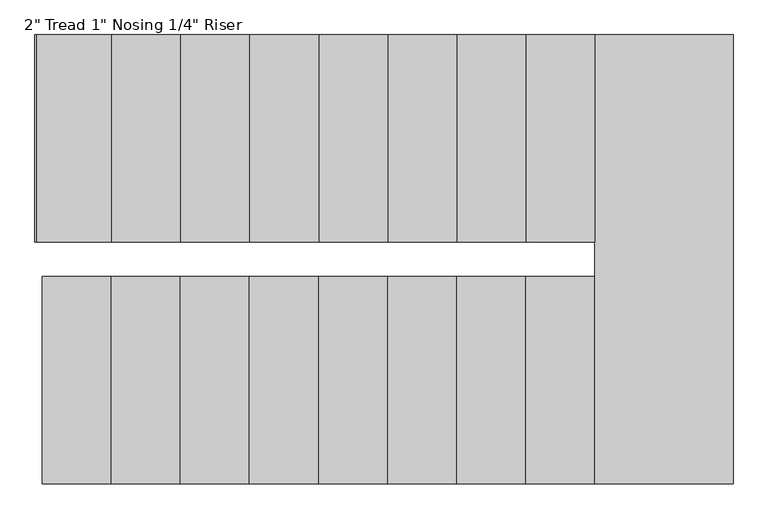
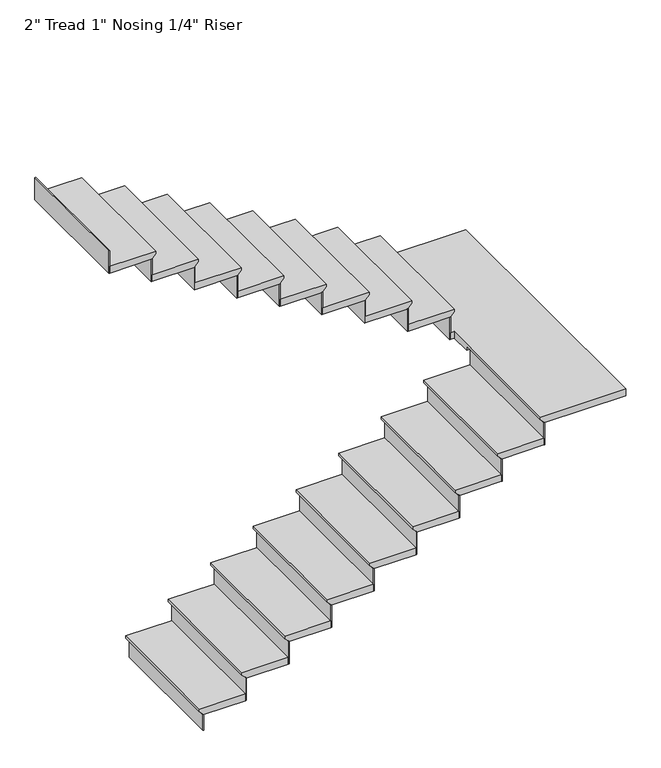
"""IFC4 building model written with IfcOpenShell, lengths in millimetres: stair flight geometry."""

from ifc_helpers import new_model, si_unit, origin, place, context, project, spatial, faceted_brep, source, transform, mapped, element, save


def stair_flight_3ef849b5(model_context):
    return source(origin(), model_context, "Body", "Brep", [
        faceted_brep([(-1197.97188, -4816.50869, 15999.8833333), (-1197.97188, -4816.50869, 16018.9333333), (-1197.97188, -3902.10869, 16018.9333333), (-1197.97188, -3902.10869, 15999.8833333), (-1172.57188, -4816.50869, 15974.4833333), (-1172.57188, -3902.10869, 15974.4833333), (-867.77188, -4816.50869, 16018.9333333), (-867.77188, -3902.10869, 16018.9333333), (-1172.57188, -3902.10869, 15968.1333333), (-867.77188, -3902.10869, 15968.1333333), (-867.77188, -4816.50869, 15968.1333333), (-1172.57188, -4816.50869, 15968.1333333)], [[[0, 1, 2, 3]], [[4, 0, 3, 5]], [[2, 1, 6, 7]], [[8, 9, 10, 11]], [[2, 7, 9, 8, 5, 3]], [[8, 11, 4, 5]], [[6, 1, 0, 4, 11, 10]], [[7, 6, 10, 9]]]),
        faceted_brep([(-1172.57188, -4816.50869, 15968.1333333), (-1172.57188, -4816.50869, 15849.6), (-1166.22188, -4816.50869, 15849.6), (-1166.22188, -4816.50869, 15968.1333333), (-1172.57188, -3902.10869, 15968.1333333), (-1166.22188, -3902.10869, 15968.1333333), (-1166.22188, -3902.10869, 15849.6), (-1172.57188, -3902.10869, 15849.6)], [[[0, 1, 2, 3]], [[4, 5, 6, 7]], [[1, 0, 4, 7]], [[2, 1, 7, 6]], [[3, 2, 6, 5]], [[0, 3, 5, 4]]]),
        faceted_brep([(-867.77188, -4816.50869, 16137.4666667), (-867.77188, -4816.50869, 15968.1333333), (-861.42188, -4816.50869, 15968.1333333), (-861.42188, -4816.50869, 16137.4666667), (-867.77188, -3902.10869, 16137.4666667), (-861.42188, -3902.10869, 16137.4666667), (-861.42188, -3902.10869, 15968.1333333), (-867.77188, -3902.10869, 15968.1333333)], [[[0, 1, 2, 3]], [[4, 5, 6, 7]], [[1, 0, 4, 7]], [[2, 1, 7, 6]], [[3, 2, 6, 5]], [[0, 3, 5, 4]]]),
        faceted_brep([(-893.17188, -3902.10869, 16188.2666667), (-893.17188, -4816.50869, 16188.2666667), (-562.97188, -4816.50869, 16188.2666667), (-562.97188, -3902.10869, 16188.2666667), (-867.77188, -3902.10869, 16137.4666667), (-562.97188, -3902.10869, 16137.4666667), (-562.97188, -4816.50869, 16137.4666667), (-867.77188, -4816.50869, 16137.4666667), (-867.77188, -3902.10869, 16143.8166667), (-893.17188, -3902.10869, 16169.2166667), (-867.77188, -4816.50869, 16143.8166667), (-893.17188, -4816.50869, 16169.2166667)], [[[0, 1, 2, 3]], [[4, 5, 6, 7]], [[0, 3, 5, 4, 8, 9]], [[4, 7, 10, 8]], [[2, 1, 11, 10, 7, 6]], [[3, 2, 6, 5]], [[11, 1, 0, 9]], [[10, 11, 9, 8]]]),
        faceted_brep([(-562.97188, -4816.50869, 16306.8), (-562.97188, -4816.50869, 16137.4666667), (-556.62188, -4816.50869, 16137.4666667), (-556.62188, -4816.50869, 16306.8), (-562.97188, -3902.10869, 16306.8), (-556.62188, -3902.10869, 16306.8), (-556.62188, -3902.10869, 16137.4666667), (-562.97188, -3902.10869, 16137.4666667)], [[[0, 1, 2, 3]], [[4, 5, 6, 7]], [[1, 0, 4, 7]], [[2, 1, 7, 6]], [[3, 2, 6, 5]], [[0, 3, 5, 4]]]),
        faceted_brep([(-588.37188, -3902.10869, 16357.6), (-588.37188, -4816.50869, 16357.6), (-258.17188, -4816.50869, 16357.6), (-258.17188, -3902.10869, 16357.6), (-562.97188, -3902.10869, 16306.8), (-258.17188, -3902.10869, 16306.8), (-258.17188, -4816.50869, 16306.8), (-562.97188, -4816.50869, 16306.8), (-562.97188, -3902.10869, 16313.15), (-588.37188, -3902.10869, 16338.55), (-562.97188, -4816.50869, 16313.15), (-588.37188, -4816.50869, 16338.55)], [[[0, 1, 2, 3]], [[4, 5, 6, 7]], [[0, 3, 5, 4, 8, 9]], [[4, 7, 10, 8]], [[2, 1, 11, 10, 7, 6]], [[3, 2, 6, 5]], [[11, 1, 0, 9]], [[10, 11, 9, 8]]]),
        faceted_brep([(-258.17188, -4816.50869, 16476.1333333), (-258.17188, -4816.50869, 16306.8), (-251.82188, -4816.50869, 16306.8), (-251.82188, -4816.50869, 16476.1333333), (-258.17188, -3902.10869, 16476.1333333), (-251.82188, -3902.10869, 16476.1333333), (-251.82188, -3902.10869, 16306.8), (-258.17188, -3902.10869, 16306.8)], [[[0, 1, 2, 3]], [[4, 5, 6, 7]], [[1, 0, 4, 7]], [[2, 1, 7, 6]], [[3, 2, 6, 5]], [[0, 3, 5, 4]]]),
        faceted_brep([(-283.57188, -3902.10869, 16526.9333333), (-283.57188, -4816.50869, 16526.9333333), (46.62812, -4816.50869, 16526.9333333), (46.62812, -3902.10869, 16526.9333333), (-258.17188, -3902.10869, 16476.1333333), (46.62812, -3902.10869, 16476.1333333), (46.62812, -4816.50869, 16476.1333333), (-258.17188, -4816.50869, 16476.1333333), (-258.17188, -3902.10869, 16482.4833333), (-283.57188, -3902.10869, 16507.8833333), (-258.17188, -4816.50869, 16482.4833333), (-283.57188, -4816.50869, 16507.8833333)], [[[0, 1, 2, 3]], [[4, 5, 6, 7]], [[0, 3, 5, 4, 8, 9]], [[4, 7, 10, 8]], [[2, 1, 11, 10, 7, 6]], [[3, 2, 6, 5]], [[11, 1, 0, 9]], [[10, 11, 9, 8]]]),
        faceted_brep([(46.62812, -4816.50869, 16645.4666667), (46.62812, -4816.50869, 16476.1333333), (52.97812, -4816.50869, 16476.1333333), (52.97812, -4816.50869, 16645.4666667), (46.62812, -3902.10869, 16645.4666667), (52.97812, -3902.10869, 16645.4666667), (52.97812, -3902.10869, 16476.1333333), (46.62812, -3902.10869, 16476.1333333)], [[[0, 1, 2, 3]], [[4, 5, 6, 7]], [[1, 0, 4, 7]], [[2, 1, 7, 6]], [[3, 2, 6, 5]], [[0, 3, 5, 4]]]),
        faceted_brep([(21.22812, -3902.10869, 16696.2666667), (21.22812, -4816.50869, 16696.2666667), (351.42812, -4816.50869, 16696.2666667), (351.42812, -3902.10869, 16696.2666667), (46.62812, -3902.10869, 16645.4666667), (351.42812, -3902.10869, 16645.4666667), (351.42812, -4816.50869, 16645.4666667), (46.62812, -4816.50869, 16645.4666667), (46.62812, -3902.10869, 16651.8166667), (21.22812, -3902.10869, 16677.2166667), (46.62812, -4816.50869, 16651.8166667), (21.22812, -4816.50869, 16677.2166667)], [[[0, 1, 2, 3]], [[4, 5, 6, 7]], [[0, 3, 5, 4, 8, 9]], [[4, 7, 10, 8]], [[2, 1, 11, 10, 7, 6]], [[3, 2, 6, 5]], [[11, 1, 0, 9]], [[10, 11, 9, 8]]]),
        faceted_brep([(351.42812, -4816.50869, 16814.8), (351.42812, -4816.50869, 16645.4666667), (357.77812, -4816.50869, 16645.4666667), (357.77812, -4816.50869, 16814.8), (351.42812, -3902.10869, 16814.8), (357.77812, -3902.10869, 16814.8), (357.77812, -3902.10869, 16645.4666667), (351.42812, -3902.10869, 16645.4666667)], [[[0, 1, 2, 3]], [[4, 5, 6, 7]], [[1, 0, 4, 7]], [[2, 1, 7, 6]], [[3, 2, 6, 5]], [[0, 3, 5, 4]]]),
        faceted_brep([(326.02812, -3902.10869, 16865.6), (326.02812, -4816.50869, 16865.6), (656.22812, -4816.50869, 16865.6), (656.22812, -3902.10869, 16865.6), (351.42812, -3902.10869, 16814.8), (656.22812, -3902.10869, 16814.8), (656.22812, -4816.50869, 16814.8), (351.42812, -4816.50869, 16814.8), (351.42812, -3902.10869, 16821.15), (326.02812, -3902.10869, 16846.55), (351.42812, -4816.50869, 16821.15), (326.02812, -4816.50869, 16846.55)], [[[0, 1, 2, 3]], [[4, 5, 6, 7]], [[0, 3, 5, 4, 8, 9]], [[4, 7, 10, 8]], [[2, 1, 11, 10, 7, 6]], [[3, 2, 6, 5]], [[11, 1, 0, 9]], [[10, 11, 9, 8]]]),
        faceted_brep([(656.22812, -4816.50869, 16984.1333333), (656.22812, -4816.50869, 16814.8), (662.57812, -4816.50869, 16814.8), (662.57812, -4816.50869, 16984.1333333), (656.22812, -3902.10869, 16984.1333333), (662.57812, -3902.10869, 16984.1333333), (662.57812, -3902.10869, 16814.8), (656.22812, -3902.10869, 16814.8)], [[[0, 1, 2, 3]], [[4, 5, 6, 7]], [[1, 0, 4, 7]], [[2, 1, 7, 6]], [[3, 2, 6, 5]], [[0, 3, 5, 4]]]),
        faceted_brep([(630.82812, -3902.10869, 17034.9333333), (630.82812, -4816.50869, 17034.9333333), (961.02812, -4816.50869, 17034.9333333), (961.02812, -3902.10869, 17034.9333333), (656.22812, -3902.10869, 16984.1333333), (961.02812, -3902.10869, 16984.1333333), (961.02812, -4816.50869, 16984.1333333), (656.22812, -4816.50869, 16984.1333333), (656.22812, -3902.10869, 16990.4833333), (630.82812, -3902.10869, 17015.8833333), (656.22812, -4816.50869, 16990.4833333), (630.82812, -4816.50869, 17015.8833333)], [[[0, 1, 2, 3]], [[4, 5, 6, 7]], [[0, 3, 5, 4, 8, 9]], [[4, 7, 10, 8]], [[2, 1, 11, 10, 7, 6]], [[3, 2, 6, 5]], [[11, 1, 0, 9]], [[10, 11, 9, 8]]]),
        faceted_brep([(961.02812, -4816.50869, 17153.4666667), (961.02812, -4816.50869, 16984.1333333), (967.37812, -4816.50869, 16984.1333333), (967.37812, -4816.50869, 17153.4666667), (961.02812, -3902.10869, 17153.4666667), (967.37812, -3902.10869, 17153.4666667), (967.37812, -3902.10869, 16984.1333333), (961.02812, -3902.10869, 16984.1333333)], [[[0, 1, 2, 3]], [[4, 5, 6, 7]], [[1, 0, 4, 7]], [[2, 1, 7, 6]], [[3, 2, 6, 5]], [[0, 3, 5, 4]]]),
        faceted_brep([(935.62812, -3902.10869, 17204.2666667), (935.62812, -4816.50869, 17204.2666667), (1265.82812, -4816.50869, 17204.2666667), (1265.82812, -3902.10869, 17204.2666667), (961.02812, -3902.10869, 17153.4666667), (1265.82812, -3902.10869, 17153.4666667), (1265.82812, -4816.50869, 17153.4666667), (961.02812, -4816.50869, 17153.4666667), (961.02812, -3902.10869, 17159.8166667), (935.62812, -3902.10869, 17185.2166667), (961.02812, -4816.50869, 17159.8166667), (935.62812, -4816.50869, 17185.2166667)], [[[0, 1, 2, 3]], [[4, 5, 6, 7]], [[0, 3, 5, 4, 8, 9]], [[4, 7, 10, 8]], [[2, 1, 11, 10, 7, 6]], [[3, 2, 6, 5]], [[11, 1, 0, 9]], [[10, 11, 9, 8]]]),
        faceted_brep([(1265.82812, -4816.50869, 17322.8), (1265.82812, -4816.50869, 17153.4666667), (1272.17812, -4816.50869, 17153.4666667), (1272.17812, -4816.50869, 17322.8), (1265.82812, -3902.10869, 17322.8), (1272.17812, -3902.10869, 17322.8), (1272.17812, -3902.10869, 17153.4666667), (1265.82812, -3902.10869, 17153.4666667)], [[[0, 1, 2, 3]], [[4, 5, 6, 7]], [[1, 0, 4, 7]], [[2, 1, 7, 6]], [[3, 2, 6, 5]], [[0, 3, 5, 4]]]),
        faceted_brep([(1215.02812, -3749.70869, 17373.6), (1240.42812, -3749.70869, 17373.6), (1240.42812, -4816.50869, 17373.6), (1850.02812, -4816.50869, 17373.6), (1850.02812, -2835.30869, 17373.6), (1215.02812, -2835.30869, 17373.6), (1240.42812, -3749.70869, 17322.8), (1215.02812, -3749.70869, 17322.8), (1215.02812, -2835.30869, 17322.8), (1850.02812, -2835.30869, 17322.8), (1850.02812, -4816.50869, 17322.8), (1265.82812, -4816.50869, 17322.8), (1265.82812, -3902.10869, 17322.8), (1240.42812, -3902.10869, 17322.8), (1240.42812, -3902.10869, 17354.55), (1240.42812, -4816.50869, 17354.55), (1265.82812, -3902.10869, 17329.15), (1265.82812, -4816.50869, 17329.15)], [[[0, 1, 2, 3, 4, 5]], [[6, 7, 8, 9, 10, 11, 12, 13]], [[1, 0, 7, 6]], [[2, 1, 6, 13, 14, 15]], [[13, 12, 16, 14]], [[12, 11, 17, 16]], [[3, 2, 15, 17, 11, 10]], [[4, 3, 10, 9]], [[5, 4, 9, 8]], [[0, 5, 8, 7]], [[17, 15, 14, 16]]]),
        faceted_brep([(1215.02812, -2835.30869, 17492.1333333), (1215.02812, -2835.30869, 17322.8), (1208.67812, -2835.30869, 17322.8), (1208.67812, -2835.30869, 17492.1333333), (1215.02812, -3749.70869, 17492.1333333), (1208.67812, -3749.70869, 17492.1333333), (1208.67812, -3749.70869, 17322.8), (1215.02812, -3749.70869, 17322.8)], [[[0, 1, 2, 3]], [[4, 5, 6, 7]], [[1, 0, 4, 7]], [[2, 1, 7, 6]], [[3, 2, 6, 5]], [[0, 3, 5, 4]]]),
        faceted_brep([(1240.42812, -3749.70869, 17542.9333333), (1240.42812, -2835.30869, 17542.9333333), (910.22812, -2835.30869, 17542.9333333), (910.22812, -3749.70869, 17542.9333333), (1215.02812, -3749.70869, 17492.1333333), (910.22812, -3749.70869, 17492.1333333), (910.22812, -2835.30869, 17492.1333333), (1215.02812, -2835.30869, 17492.1333333), (1215.02812, -3749.70869, 17498.4833333), (1240.42812, -3749.70869, 17523.8833333), (1215.02812, -2835.30869, 17498.4833333), (1240.42812, -2835.30869, 17523.8833333)], [[[0, 1, 2, 3]], [[4, 5, 6, 7]], [[0, 3, 5, 4, 8, 9]], [[4, 7, 10, 8]], [[2, 1, 11, 10, 7, 6]], [[3, 2, 6, 5]], [[11, 1, 0, 9]], [[10, 11, 9, 8]]]),
        faceted_brep([(910.22812, -2835.30869, 17661.4666667), (910.22812, -2835.30869, 17492.1333333), (903.87812, -2835.30869, 17492.1333333), (903.87812, -2835.30869, 17661.4666667), (910.22812, -3749.70869, 17661.4666667), (903.87812, -3749.70869, 17661.4666667), (903.87812, -3749.70869, 17492.1333333), (910.22812, -3749.70869, 17492.1333333)], [[[0, 1, 2, 3]], [[4, 5, 6, 7]], [[1, 0, 4, 7]], [[2, 1, 7, 6]], [[3, 2, 6, 5]], [[0, 3, 5, 4]]]),
        faceted_brep([(935.62812, -3749.70869, 17712.2666667), (935.62812, -2835.30869, 17712.2666667), (605.42812, -2835.30869, 17712.2666667), (605.42812, -3749.70869, 17712.2666667), (910.22812, -3749.70869, 17661.4666667), (605.42812, -3749.70869, 17661.4666667), (605.42812, -2835.30869, 17661.4666667), (910.22812, -2835.30869, 17661.4666667), (910.22812, -3749.70869, 17667.8166667), (935.62812, -3749.70869, 17693.2166667), (910.22812, -2835.30869, 17667.8166667), (935.62812, -2835.30869, 17693.2166667)], [[[0, 1, 2, 3]], [[4, 5, 6, 7]], [[0, 3, 5, 4, 8, 9]], [[4, 7, 10, 8]], [[2, 1, 11, 10, 7, 6]], [[3, 2, 6, 5]], [[11, 1, 0, 9]], [[10, 11, 9, 8]]]),
        faceted_brep([(605.42812, -2835.30869, 17830.8), (605.42812, -2835.30869, 17661.4666667), (599.07812, -2835.30869, 17661.4666667), (599.07812, -2835.30869, 17830.8), (605.42812, -3749.70869, 17830.8), (599.07812, -3749.70869, 17830.8), (599.07812, -3749.70869, 17661.4666667), (605.42812, -3749.70869, 17661.4666667)], [[[0, 1, 2, 3]], [[4, 5, 6, 7]], [[1, 0, 4, 7]], [[2, 1, 7, 6]], [[3, 2, 6, 5]], [[0, 3, 5, 4]]]),
        faceted_brep([(630.82812, -3749.70869, 17881.6), (630.82812, -2835.30869, 17881.6), (300.62812, -2835.30869, 17881.6), (300.62812, -3749.70869, 17881.6), (605.42812, -3749.70869, 17830.8), (300.62812, -3749.70869, 17830.8), (300.62812, -2835.30869, 17830.8), (605.42812, -2835.30869, 17830.8), (605.42812, -3749.70869, 17837.15), (630.82812, -3749.70869, 17862.55), (605.42812, -2835.30869, 17837.15), (630.82812, -2835.30869, 17862.55)], [[[0, 1, 2, 3]], [[4, 5, 6, 7]], [[0, 3, 5, 4, 8, 9]], [[4, 7, 10, 8]], [[2, 1, 11, 10, 7, 6]], [[3, 2, 6, 5]], [[11, 1, 0, 9]], [[10, 11, 9, 8]]]),
        faceted_brep([(300.62812, -2835.30869, 18000.1333333), (300.62812, -2835.30869, 17830.8), (294.27812, -2835.30869, 17830.8), (294.27812, -2835.30869, 18000.1333333), (300.62812, -3749.70869, 18000.1333333), (294.27812, -3749.70869, 18000.1333333), (294.27812, -3749.70869, 17830.8), (300.62812, -3749.70869, 17830.8)], [[[0, 1, 2, 3]], [[4, 5, 6, 7]], [[1, 0, 4, 7]], [[2, 1, 7, 6]], [[3, 2, 6, 5]], [[0, 3, 5, 4]]]),
        faceted_brep([(326.02812, -3749.70869, 18050.9333333), (326.02812, -2835.30869, 18050.9333333), (-4.17188, -2835.30869, 18050.9333333), (-4.17188, -3749.70869, 18050.9333333), (300.62812, -3749.70869, 18000.1333333), (-4.17188, -3749.70869, 18000.1333333), (-4.17188, -2835.30869, 18000.1333333), (300.62812, -2835.30869, 18000.1333333), (300.62812, -3749.70869, 18006.4833333), (326.02812, -3749.70869, 18031.8833333), (300.62812, -2835.30869, 18006.4833333), (326.02812, -2835.30869, 18031.8833333)], [[[0, 1, 2, 3]], [[4, 5, 6, 7]], [[0, 3, 5, 4, 8, 9]], [[4, 7, 10, 8]], [[2, 1, 11, 10, 7, 6]], [[3, 2, 6, 5]], [[11, 1, 0, 9]], [[10, 11, 9, 8]]]),
        faceted_brep([(-4.17188, -2835.30869, 18169.4666667), (-4.17188, -2835.30869, 18000.1333333), (-10.52188, -2835.30869, 18000.1333333), (-10.52188, -2835.30869, 18169.4666667), (-4.17188, -3749.70869, 18169.4666667), (-10.52188, -3749.70869, 18169.4666667), (-10.52188, -3749.70869, 18000.1333333), (-4.17188, -3749.70869, 18000.1333333)], [[[0, 1, 2, 3]], [[4, 5, 6, 7]], [[1, 0, 4, 7]], [[2, 1, 7, 6]], [[3, 2, 6, 5]], [[0, 3, 5, 4]]]),
        faceted_brep([(21.22812, -3749.70869, 18220.2666667), (21.22812, -2835.30869, 18220.2666667), (-308.97188, -2835.30869, 18220.2666667), (-308.97188, -3749.70869, 18220.2666667), (-4.17188, -3749.70869, 18169.4666667), (-308.97188, -3749.70869, 18169.4666667), (-308.97188, -2835.30869, 18169.4666667), (-4.17188, -2835.30869, 18169.4666667), (-4.17188, -3749.70869, 18175.8166667), (21.22812, -3749.70869, 18201.2166667), (-4.17188, -2835.30869, 18175.8166667), (21.22812, -2835.30869, 18201.2166667)], [[[0, 1, 2, 3]], [[4, 5, 6, 7]], [[0, 3, 5, 4, 8, 9]], [[4, 7, 10, 8]], [[2, 1, 11, 10, 7, 6]], [[3, 2, 6, 5]], [[11, 1, 0, 9]], [[10, 11, 9, 8]]]),
        faceted_brep([(-308.97188, -2835.30869, 18338.8), (-308.97188, -2835.30869, 18169.4666667), (-315.32188, -2835.30869, 18169.4666667), (-315.32188, -2835.30869, 18338.8), (-308.97188, -3749.70869, 18338.8), (-315.32188, -3749.70869, 18338.8), (-315.32188, -3749.70869, 18169.4666667), (-308.97188, -3749.70869, 18169.4666667)], [[[0, 1, 2, 3]], [[4, 5, 6, 7]], [[1, 0, 4, 7]], [[2, 1, 7, 6]], [[3, 2, 6, 5]], [[0, 3, 5, 4]]]),
        faceted_brep([(-283.57188, -3749.70869, 18389.6), (-283.57188, -2835.30869, 18389.6), (-613.77188, -2835.30869, 18389.6), (-613.77188, -3749.70869, 18389.6), (-308.97188, -3749.70869, 18338.8), (-613.77188, -3749.70869, 18338.8), (-613.77188, -2835.30869, 18338.8), (-308.97188, -2835.30869, 18338.8), (-308.97188, -3749.70869, 18345.15), (-283.57188, -3749.70869, 18370.55), (-308.97188, -2835.30869, 18345.15), (-283.57188, -2835.30869, 18370.55)], [[[0, 1, 2, 3]], [[4, 5, 6, 7]], [[0, 3, 5, 4, 8, 9]], [[4, 7, 10, 8]], [[2, 1, 11, 10, 7, 6]], [[3, 2, 6, 5]], [[11, 1, 0, 9]], [[10, 11, 9, 8]]]),
        faceted_brep([(-613.77188, -2835.30869, 18508.1333333), (-613.77188, -2835.30869, 18338.8), (-620.12188, -2835.30869, 18338.8), (-620.12188, -2835.30869, 18508.1333333), (-613.77188, -3749.70869, 18508.1333333), (-620.12188, -3749.70869, 18508.1333333), (-620.12188, -3749.70869, 18338.8), (-613.77188, -3749.70869, 18338.8)], [[[0, 1, 2, 3]], [[4, 5, 6, 7]], [[1, 0, 4, 7]], [[2, 1, 7, 6]], [[3, 2, 6, 5]], [[0, 3, 5, 4]]]),
        faceted_brep([(-588.37188, -3749.70869, 18558.9333333), (-588.37188, -2835.30869, 18558.9333333), (-918.57188, -2835.30869, 18558.9333333), (-918.57188, -3749.70869, 18558.9333333), (-613.77188, -3749.70869, 18508.1333333), (-918.57188, -3749.70869, 18508.1333333), (-918.57188, -2835.30869, 18508.1333333), (-613.77188, -2835.30869, 18508.1333333), (-613.77188, -3749.70869, 18514.4833333), (-588.37188, -3749.70869, 18539.8833333), (-613.77188, -2835.30869, 18514.4833333), (-588.37188, -2835.30869, 18539.8833333)], [[[0, 1, 2, 3]], [[4, 5, 6, 7]], [[0, 3, 5, 4, 8, 9]], [[4, 7, 10, 8]], [[2, 1, 11, 10, 7, 6]], [[3, 2, 6, 5]], [[11, 1, 0, 9]], [[10, 11, 9, 8]]]),
        faceted_brep([(-918.57188, -2835.30869, 18677.4666667), (-918.57188, -2835.30869, 18508.1333333), (-924.92188, -2835.30869, 18508.1333333), (-924.92188, -2835.30869, 18677.4666667), (-918.57188, -3749.70869, 18677.4666667), (-924.92188, -3749.70869, 18677.4666667), (-924.92188, -3749.70869, 18508.1333333), (-918.57188, -3749.70869, 18508.1333333)], [[[0, 1, 2, 3]], [[4, 5, 6, 7]], [[1, 0, 4, 7]], [[2, 1, 7, 6]], [[3, 2, 6, 5]], [[0, 3, 5, 4]]]),
        faceted_brep([(-1223.37188, -2835.30869, 18846.8), (-1223.37188, -2835.30869, 18677.4666667), (-1229.72188, -2835.30869, 18677.4666667), (-1229.72188, -2835.30869, 18846.8), (-1223.37188, -3749.70869, 18846.8), (-1229.72188, -3749.70869, 18846.8), (-1229.72188, -3749.70869, 18677.4666667), (-1223.37188, -3749.70869, 18677.4666667)], [[[0, 1, 2, 3]], [[4, 5, 6, 7]], [[1, 0, 4, 7]], [[2, 1, 7, 6]], [[3, 2, 6, 5]], [[0, 3, 5, 4]]]),
        faceted_brep([(-893.17188, -3749.70869, 18728.2666667), (-893.17188, -2835.30869, 18728.2666667), (-1223.37188, -2835.30869, 18728.2666667), (-1223.37188, -3749.70869, 18728.2666667), (-918.57188, -3749.70869, 18677.4666667), (-1223.37188, -3749.70869, 18677.4666667), (-1223.37188, -2835.30869, 18677.4666667), (-918.57188, -2835.30869, 18677.4666667), (-918.57188, -3749.70869, 18683.8166667), (-893.17188, -3749.70869, 18709.2166667), (-918.57188, -2835.30869, 18683.8166667), (-893.17188, -2835.30869, 18709.2166667)], [[[0, 1, 2, 3]], [[4, 5, 6, 7]], [[0, 3, 5, 4, 8, 9]], [[4, 7, 10, 8]], [[2, 1, 11, 10, 7, 6]], [[3, 2, 6, 5]], [[11, 1, 0, 9]], [[10, 11, 9, 8]]]),
    ])


if __name__ == "__main__":
    model = new_model("IFC4")
    model_context = context("Model", 3, world=origin())
    ifc_project = project(units=[si_unit("LENGTHUNIT", "METRE", prefix="MILLI")], contexts=[model_context])
    site = spatial("IfcSite", under=ifc_project)
    building = spatial("IfcBuilding", under=site)
    placement = place(None, origin())
    stair_flight_shape = stair_flight_3ef849b5(model_context)
    element("IfcStairFlight", 1, ObjectType="2\" Tread 1\" Nosing 1/4\" Riser", at=placement, inside=building, context=model_context, shape_type="MappedRepresentation", body=[
        mapped(stair_flight_shape, transform((0.0, 0.0, 0.0), x_axis=(1.0, 0.0, 0.0), y_axis=(0.0, 1.0, 0.0), z_axis=(0.0, 0.0, 1.0))),
    ])
    save(model, "model.ifc")
